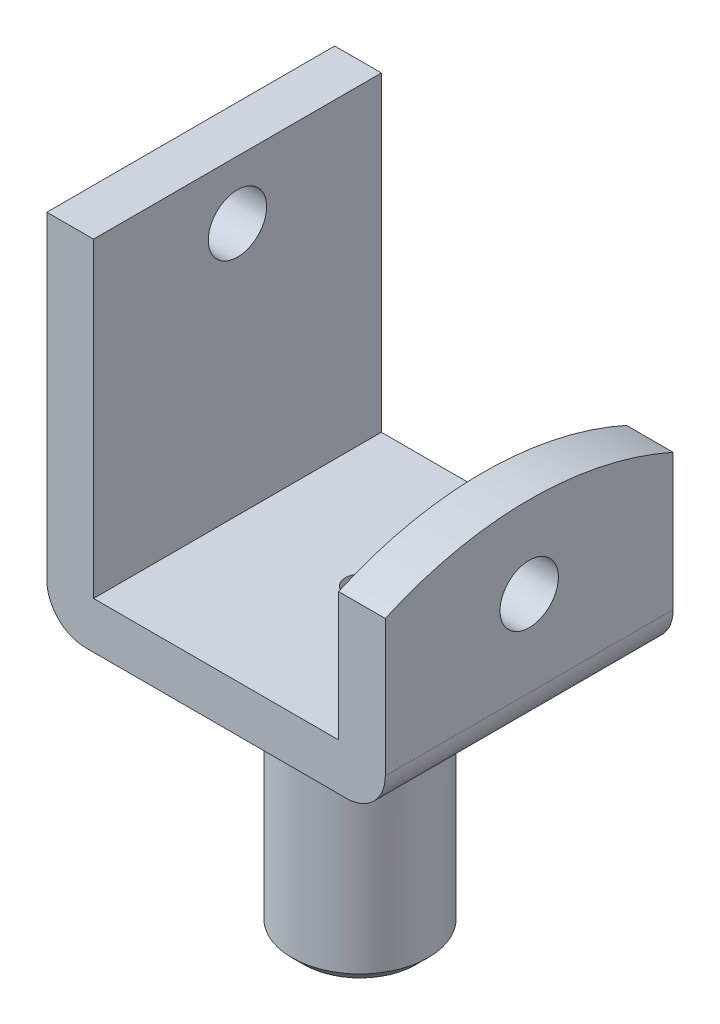
ISO-10303-21;
HEADER;
FILE_DESCRIPTION(('STEP AP214'),'2;1');
FILE_NAME('part.step','',(''),(''),'','','');
FILE_SCHEMA(('AUTOMOTIVE_DESIGN { 1 0 10303 214 1 1 1 1 }'));
ENDSEC;
DATA;
#1=APPLICATION_CONTEXT('core data for automotive mechanical design processes');
#2=APPLICATION_PROTOCOL_DEFINITION('international standard','automotive_design',2000,#1);
#3=PRODUCT_CONTEXT('',#1,'mechanical');
#4=PRODUCT('Part','Part','',(#3));
#5=PRODUCT_RELATED_PRODUCT_CATEGORY('part','',(#4));
#6=PRODUCT_DEFINITION_FORMATION('','',#4);
#7=PRODUCT_DEFINITION_CONTEXT('part definition',#1,'design');
#8=PRODUCT_DEFINITION('design','',#6,#7);
#9=PRODUCT_DEFINITION_SHAPE('','',#8);
#10=(LENGTH_UNIT() NAMED_UNIT(*) SI_UNIT(.MILLI.,.METRE.));
#11=(NAMED_UNIT(*) PLANE_ANGLE_UNIT() SI_UNIT($,.RADIAN.));
#12=(NAMED_UNIT(*) SI_UNIT($,.STERADIAN.) SOLID_ANGLE_UNIT());
#13=UNCERTAINTY_MEASURE_WITH_UNIT(LENGTH_MEASURE(1.E-05),#10,'distance_accuracy_value','');
#14=(GEOMETRIC_REPRESENTATION_CONTEXT(3) GLOBAL_UNCERTAINTY_ASSIGNED_CONTEXT((#13)) GLOBAL_UNIT_ASSIGNED_CONTEXT((#10,
#11,#12)) REPRESENTATION_CONTEXT('',''));
#15=CARTESIAN_POINT('',(0.,0.,0.));
#16=DIRECTION('',(0.,0.,1.));
#17=DIRECTION('',(1.,0.,0.));
#18=AXIS2_PLACEMENT_3D('',#15,#16,#17);
#19=CARTESIAN_POINT('',(43500.,6000.,37000.));
#20=DIRECTION('',(-1.,0.,0.));
#21=DIRECTION('',(0.,-1.,0.));
#22=AXIS2_PLACEMENT_3D('',#19,#20,#21);
#23=PLANE('',#22);
#24=CARTESIAN_POINT('',(43500.,26000.,-2.57175827820944E-12));
#25=DIRECTION('',(1.,0.,0.));
#26=DIRECTION('',(0.,1.,0.));
#27=AXIS2_PLACEMENT_3D('',#24,#25,#26);
#28=CIRCLE('',#27,7500.);
#29=CARTESIAN_POINT('',(43500.,33500.,-2.57175827820944E-12));
#30=VERTEX_POINT('',#29);
#31=EDGE_CURVE('E264',#30,#30,#28,.T.);
#32=ORIENTED_EDGE('',*,*,#31,.F.);
#33=EDGE_LOOP('',(#32));
#34=FACE_BOUND('',#33,.T.);
#35=CARTESIAN_POINT('',(43500.,-43000.,-1.10218211923262E-11));
#36=DIRECTION('',(1.,0.,0.));
#37=DIRECTION('',(0.,1.,0.));
#38=AXIS2_PLACEMENT_3D('',#35,#36,#37);
#39=CIRCLE('',#38,90000.);
#40=CARTESIAN_POINT('',(43500.,39042.6718238747,-37000.));
#41=VERTEX_POINT('',#40);
#42=CARTESIAN_POINT('',(43500.,39042.6718238747,37000.));
#43=VERTEX_POINT('',#42);
#44=EDGE_CURVE('E61',#41,#43,#39,.T.);
#45=ORIENTED_EDGE('',*,*,#44,.T.);
#46=DIRECTION('',(0.,1.,0.));
#47=VECTOR('',#46,1.);
#48=CARTESIAN_POINT('',(43500.,6000.,37000.));
#49=LINE('',#48,#47);
#50=CARTESIAN_POINT('',(43500.,4000.,37000.));
#51=VERTEX_POINT('',#50);
#52=EDGE_CURVE('E142',#51,#43,#49,.T.);
#53=ORIENTED_EDGE('',*,*,#52,.F.);
#54=DIRECTION('',(0.,0.,-1.));
#55=VECTOR('',#54,1.);
#56=CARTESIAN_POINT('',(43500.,4000.,37000.));
#57=LINE('',#56,#55);
#58=CARTESIAN_POINT('',(43500.,4000.,-37000.));
#59=VERTEX_POINT('',#58);
#60=EDGE_CURVE('E187',#51,#59,#57,.T.);
#61=ORIENTED_EDGE('',*,*,#60,.T.);
#62=DIRECTION('',(0.,1.,0.));
#63=VECTOR('',#62,1.);
#64=CARTESIAN_POINT('',(43500.,6000.,-37000.));
#65=LINE('',#64,#63);
#66=EDGE_CURVE('E162',#59,#41,#65,.T.);
#67=ORIENTED_EDGE('',*,*,#66,.T.);
#68=EDGE_LOOP('',(#45,#53,#61,#67));
#69=FACE_BOUND('',#68,.T.);
#70=ADVANCED_FACE('F48',(#34,#69),#23,.F.);
#71=CARTESIAN_POINT('',(31500.,6000.,37000.));
#72=DIRECTION('',(1.,0.,0.));
#73=DIRECTION('',(0.,0.,-1.));
#74=AXIS2_PLACEMENT_3D('',#71,#72,#73);
#75=PLANE('',#74);
#76=CARTESIAN_POINT('',(31500.,26000.,-2.57175827820944E-12));
#77=DIRECTION('',(1.,0.,0.));
#78=DIRECTION('',(0.,1.,0.));
#79=AXIS2_PLACEMENT_3D('',#76,#77,#78);
#80=CIRCLE('',#79,7500.);
#81=CARTESIAN_POINT('',(31500.,33500.,-2.57175827820944E-12));
#82=VERTEX_POINT('',#81);
#83=EDGE_CURVE('E263',#82,#82,#80,.T.);
#84=ORIENTED_EDGE('',*,*,#83,.T.);
#85=EDGE_LOOP('',(#84));
#86=FACE_BOUND('',#85,.T.);
#87=CARTESIAN_POINT('',(31500.,-43000.,-1.10218211923262E-11));
#88=DIRECTION('',(1.,0.,0.));
#89=DIRECTION('',(0.,1.,0.));
#90=AXIS2_PLACEMENT_3D('',#87,#88,#89);
#91=CIRCLE('',#90,90000.);
#92=CARTESIAN_POINT('',(31500.,39042.6718238747,-37000.));
#93=VERTEX_POINT('',#92);
#94=CARTESIAN_POINT('',(31500.,39042.6718238747,37000.));
#95=VERTEX_POINT('',#94);
#96=EDGE_CURVE('E127',#93,#95,#91,.T.);
#97=ORIENTED_EDGE('',*,*,#96,.F.);
#98=DIRECTION('',(0.,-1.,0.));
#99=VECTOR('',#98,1.);
#100=CARTESIAN_POINT('',(31500.,6000.,-37000.));
#101=LINE('',#100,#99);
#102=CARTESIAN_POINT('',(31500.,6000.,-37000.));
#103=VERTEX_POINT('',#102);
#104=EDGE_CURVE('E164',#93,#103,#101,.T.);
#105=ORIENTED_EDGE('',*,*,#104,.T.);
#106=DIRECTION('',(0.,0.,-1.));
#107=VECTOR('',#106,1.);
#108=CARTESIAN_POINT('',(31500.,6000.,37000.));
#109=LINE('',#108,#107);
#110=CARTESIAN_POINT('',(31500.,6000.,37000.));
#111=VERTEX_POINT('',#110);
#112=EDGE_CURVE('E143',#111,#103,#109,.T.);
#113=ORIENTED_EDGE('',*,*,#112,.F.);
#114=DIRECTION('',(0.,-1.,0.));
#115=VECTOR('',#114,1.);
#116=CARTESIAN_POINT('',(31500.,6000.,37000.));
#117=LINE('',#116,#115);
#118=EDGE_CURVE('E140',#95,#111,#117,.T.);
#119=ORIENTED_EDGE('',*,*,#118,.F.);
#120=EDGE_LOOP('',(#97,#105,#113,#119));
#121=FACE_BOUND('',#120,.T.);
#122=ADVANCED_FACE('F141',(#86,#121),#75,.F.);
#123=CARTESIAN_POINT('',(0.,0.,37000.));
#124=DIRECTION('',(0.,0.,1.));
#125=DIRECTION('',(1.,0.,0.));
#126=AXIS2_PLACEMENT_3D('',#123,#124,#125);
#127=PLANE('',#126);
#128=ORIENTED_EDGE('',*,*,#118,.T.);
#129=DIRECTION('',(-1.,0.,0.));
#130=VECTOR('',#129,1.);
#131=CARTESIAN_POINT('',(-31500.,5999.99999999999,37000.));
#132=LINE('',#131,#130);
#133=CARTESIAN_POINT('',(-31500.,5999.99999999999,37000.));
#134=VERTEX_POINT('',#133);
#135=EDGE_CURVE('E150',#111,#134,#132,.T.);
#136=ORIENTED_EDGE('',*,*,#135,.T.);
#137=DIRECTION('',(0.,1.,0.));
#138=VECTOR('',#137,1.);
#139=CARTESIAN_POINT('',(-31500.,5999.99999999999,37000.));
#140=LINE('',#139,#138);
#141=CARTESIAN_POINT('',(-31500.,86000.,37000.));
#142=VERTEX_POINT('',#141);
#143=EDGE_CURVE('E146',#134,#142,#140,.T.);
#144=ORIENTED_EDGE('',*,*,#143,.T.);
#145=DIRECTION('',(-1.,0.,0.));
#146=VECTOR('',#145,1.);
#147=CARTESIAN_POINT('',(-43500.,86000.,37000.));
#148=LINE('',#147,#146);
#149=CARTESIAN_POINT('',(-43500.,86000.,37000.));
#150=VERTEX_POINT('',#149);
#151=EDGE_CURVE('E152',#142,#150,#148,.T.);
#152=ORIENTED_EDGE('',*,*,#151,.T.);
#153=DIRECTION('',(0.,-1.,0.));
#154=VECTOR('',#153,1.);
#155=CARTESIAN_POINT('',(-43500.,6000.,37000.));
#156=LINE('',#155,#154);
#157=CARTESIAN_POINT('',(-43500.,4000.,37000.));
#158=VERTEX_POINT('',#157);
#159=EDGE_CURVE('E159',#150,#158,#156,.T.);
#160=ORIENTED_EDGE('',*,*,#159,.T.);
#161=CARTESIAN_POINT('',(-33500.,4000.,37000.));
#162=DIRECTION('',(0.,0.,1.));
#163=DIRECTION('',(1.,0.,0.));
#164=AXIS2_PLACEMENT_3D('',#161,#162,#163);
#165=CIRCLE('',#164,10000.);
#166=CARTESIAN_POINT('',(-33500.,-6000.,37000.));
#167=VERTEX_POINT('',#166);
#168=EDGE_CURVE('E205',#158,#167,#165,.T.);
#169=ORIENTED_EDGE('',*,*,#168,.T.);
#170=DIRECTION('',(1.,0.,0.));
#171=VECTOR('',#170,1.);
#172=CARTESIAN_POINT('',(-43500.,-6000.,37000.));
#173=LINE('',#172,#171);
#174=CARTESIAN_POINT('',(33500.,-6000.,37000.));
#175=VERTEX_POINT('',#174);
#176=EDGE_CURVE('E156',#167,#175,#173,.T.);
#177=ORIENTED_EDGE('',*,*,#176,.T.);
#178=CARTESIAN_POINT('',(33500.,4000.,37000.));
#179=DIRECTION('',(0.,0.,1.));
#180=DIRECTION('',(1.,0.,0.));
#181=AXIS2_PLACEMENT_3D('',#178,#179,#180);
#182=CIRCLE('',#181,10000.);
#183=EDGE_CURVE('E193',#175,#51,#182,.T.);
#184=ORIENTED_EDGE('',*,*,#183,.T.);
#185=ORIENTED_EDGE('',*,*,#52,.T.);
#186=DIRECTION('',(1.,0.,0.));
#187=VECTOR('',#186,1.);
#188=CARTESIAN_POINT('',(31500.,39042.6718238747,37000.));
#189=LINE('',#188,#187);
#190=EDGE_CURVE('E126',#95,#43,#189,.T.);
#191=ORIENTED_EDGE('',*,*,#190,.F.);
#192=EDGE_LOOP('',(#128,#136,#144,#152,#160,#169,#177,#184,#185,#191));
#193=FACE_BOUND('',#192,.T.);
#194=ADVANCED_FACE('F139',(#193),#127,.T.);
#195=CARTESIAN_POINT('',(0.,0.,-37000.));
#196=DIRECTION('',(0.,0.,1.));
#197=DIRECTION('',(1.,0.,0.));
#198=AXIS2_PLACEMENT_3D('',#195,#196,#197);
#199=PLANE('',#198);
#200=CARTESIAN_POINT('',(33500.,4000.,-37000.));
#201=DIRECTION('',(0.,0.,1.));
#202=DIRECTION('',(1.,0.,0.));
#203=AXIS2_PLACEMENT_3D('',#200,#201,#202);
#204=CIRCLE('',#203,10000.);
#205=CARTESIAN_POINT('',(33500.,-6000.,-37000.));
#206=VERTEX_POINT('',#205);
#207=EDGE_CURVE('E186',#59,#206,#204,.F.);
#208=ORIENTED_EDGE('',*,*,#207,.T.);
#209=DIRECTION('',(1.,0.,0.));
#210=VECTOR('',#209,1.);
#211=CARTESIAN_POINT('',(-43500.,-6000.,-37000.));
#212=LINE('',#211,#210);
#213=CARTESIAN_POINT('',(-33500.,-6000.,-37000.));
#214=VERTEX_POINT('',#213);
#215=EDGE_CURVE('E153',#214,#206,#212,.T.);
#216=ORIENTED_EDGE('',*,*,#215,.F.);
#217=CARTESIAN_POINT('',(-33500.,4000.,-37000.));
#218=DIRECTION('',(0.,0.,1.));
#219=DIRECTION('',(1.,0.,0.));
#220=AXIS2_PLACEMENT_3D('',#217,#218,#219);
#221=CIRCLE('',#220,10000.);
#222=CARTESIAN_POINT('',(-43500.,4000.,-37000.));
#223=VERTEX_POINT('',#222);
#224=EDGE_CURVE('E197',#214,#223,#221,.F.);
#225=ORIENTED_EDGE('',*,*,#224,.T.);
#226=DIRECTION('',(0.,-1.,0.));
#227=VECTOR('',#226,1.);
#228=CARTESIAN_POINT('',(-43500.,6000.,-37000.));
#229=LINE('',#228,#227);
#230=CARTESIAN_POINT('',(-43500.,86000.,-37000.));
#231=VERTEX_POINT('',#230);
#232=EDGE_CURVE('E172',#231,#223,#229,.T.);
#233=ORIENTED_EDGE('',*,*,#232,.F.);
#234=DIRECTION('',(-1.,0.,0.));
#235=VECTOR('',#234,1.);
#236=CARTESIAN_POINT('',(-43500.,86000.,-37000.));
#237=LINE('',#236,#235);
#238=CARTESIAN_POINT('',(-31500.,86000.,-37000.));
#239=VERTEX_POINT('',#238);
#240=EDGE_CURVE('E171',#239,#231,#237,.T.);
#241=ORIENTED_EDGE('',*,*,#240,.F.);
#242=DIRECTION('',(0.,1.,0.));
#243=VECTOR('',#242,1.);
#244=CARTESIAN_POINT('',(-31500.,5999.99999999999,-37000.));
#245=LINE('',#244,#243);
#246=CARTESIAN_POINT('',(-31500.,5999.99999999999,-37000.));
#247=VERTEX_POINT('',#246);
#248=EDGE_CURVE('E169',#247,#239,#245,.T.);
#249=ORIENTED_EDGE('',*,*,#248,.F.);
#250=DIRECTION('',(-1.,0.,0.));
#251=VECTOR('',#250,1.);
#252=CARTESIAN_POINT('',(-31500.,5999.99999999999,-37000.));
#253=LINE('',#252,#251);
#254=EDGE_CURVE('E170',#103,#247,#253,.T.);
#255=ORIENTED_EDGE('',*,*,#254,.F.);
#256=ORIENTED_EDGE('',*,*,#104,.F.);
#257=DIRECTION('',(1.,0.,0.));
#258=VECTOR('',#257,1.);
#259=CARTESIAN_POINT('',(31500.,39042.6718238747,-37000.));
#260=LINE('',#259,#258);
#261=EDGE_CURVE('E133',#93,#41,#260,.T.);
#262=ORIENTED_EDGE('',*,*,#261,.T.);
#263=ORIENTED_EDGE('',*,*,#66,.F.);
#264=EDGE_LOOP('',(#208,#216,#225,#233,#241,#249,#255,#256,#262,#263));
#265=FACE_BOUND('',#264,.T.);
#266=ADVANCED_FACE('F266',(#265),#199,.F.);
#267=CARTESIAN_POINT('',(-31500.,5999.99999999999,37000.));
#268=DIRECTION('',(0.,-1.,0.));
#269=DIRECTION('',(1.,0.,0.));
#270=AXIS2_PLACEMENT_3D('',#267,#268,#269);
#271=PLANE('',#270);
#272=CARTESIAN_POINT('',(0.,5999.99999999999,0.));
#273=DIRECTION('',(0.,-1.,0.));
#274=DIRECTION('',(1.,0.,0.));
#275=AXIS2_PLACEMENT_3D('',#272,#273,#274);
#276=CIRCLE('',#275,3750.);
#277=CARTESIAN_POINT('',(3750.,5999.99999999999,0.));
#278=VERTEX_POINT('',#277);
#279=EDGE_CURVE('E310',#278,#278,#276,.T.);
#280=ORIENTED_EDGE('',*,*,#279,.T.);
#281=EDGE_LOOP('',(#280));
#282=FACE_BOUND('',#281,.T.);
#283=ORIENTED_EDGE('',*,*,#254,.T.);
#284=DIRECTION('',(0.,0.,-1.));
#285=VECTOR('',#284,1.);
#286=CARTESIAN_POINT('',(-31500.,5999.99999999999,37000.));
#287=LINE('',#286,#285);
#288=EDGE_CURVE('E185',#134,#247,#287,.T.);
#289=ORIENTED_EDGE('',*,*,#288,.F.);
#290=ORIENTED_EDGE('',*,*,#135,.F.);
#291=ORIENTED_EDGE('',*,*,#112,.T.);
#292=EDGE_LOOP('',(#283,#289,#290,#291));
#293=FACE_BOUND('',#292,.T.);
#294=ADVANCED_FACE('F271',(#282,#293),#271,.F.);
#295=CARTESIAN_POINT('',(-31500.,5999.99999999999,37000.));
#296=DIRECTION('',(-1.,0.,0.));
#297=DIRECTION('',(0.,0.,1.));
#298=AXIS2_PLACEMENT_3D('',#295,#296,#297);
#299=PLANE('',#298);
#300=CARTESIAN_POINT('',(-31500.,71000.,1.83697019872103E-12));
#301=DIRECTION('',(-1.,0.,0.));
#302=DIRECTION('',(0.,0.,1.));
#303=AXIS2_PLACEMENT_3D('',#300,#301,#302);
#304=CIRCLE('',#303,7500.);
#305=CARTESIAN_POINT('',(-31500.,71000.,7500.));
#306=VERTEX_POINT('',#305);
#307=EDGE_CURVE('E312',#306,#306,#304,.T.);
#308=ORIENTED_EDGE('',*,*,#307,.T.);
#309=EDGE_LOOP('',(#308));
#310=FACE_BOUND('',#309,.T.);
#311=ORIENTED_EDGE('',*,*,#248,.T.);
#312=DIRECTION('',(0.,0.,-1.));
#313=VECTOR('',#312,1.);
#314=CARTESIAN_POINT('',(-31500.,86000.,37000.));
#315=LINE('',#314,#313);
#316=EDGE_CURVE('E177',#142,#239,#315,.T.);
#317=ORIENTED_EDGE('',*,*,#316,.F.);
#318=ORIENTED_EDGE('',*,*,#143,.F.);
#319=ORIENTED_EDGE('',*,*,#288,.T.);
#320=EDGE_LOOP('',(#311,#317,#318,#319));
#321=FACE_BOUND('',#320,.T.);
#322=ADVANCED_FACE('F278',(#310,#321),#299,.F.);
#323=CARTESIAN_POINT('',(-43500.,86000.,37000.));
#324=DIRECTION('',(0.,-1.,0.));
#325=DIRECTION('',(0.,0.,-1.));
#326=AXIS2_PLACEMENT_3D('',#323,#324,#325);
#327=PLANE('',#326);
#328=ORIENTED_EDGE('',*,*,#240,.T.);
#329=DIRECTION('',(0.,0.,-1.));
#330=VECTOR('',#329,1.);
#331=CARTESIAN_POINT('',(-43500.,86000.,37000.));
#332=LINE('',#331,#330);
#333=EDGE_CURVE('E163',#150,#231,#332,.T.);
#334=ORIENTED_EDGE('',*,*,#333,.F.);
#335=ORIENTED_EDGE('',*,*,#151,.F.);
#336=ORIENTED_EDGE('',*,*,#316,.T.);
#337=EDGE_LOOP('',(#328,#334,#335,#336));
#338=FACE_BOUND('',#337,.T.);
#339=ADVANCED_FACE('F281',(#338),#327,.F.);
#340=CARTESIAN_POINT('',(-43500.,6000.,37000.));
#341=DIRECTION('',(1.,0.,0.));
#342=DIRECTION('',(0.,0.,-1.));
#343=AXIS2_PLACEMENT_3D('',#340,#341,#342);
#344=PLANE('',#343);
#345=CARTESIAN_POINT('',(-43500.,71000.,1.83697019872103E-12));
#346=DIRECTION('',(-1.,0.,0.));
#347=DIRECTION('',(0.,0.,1.));
#348=AXIS2_PLACEMENT_3D('',#345,#346,#347);
#349=CIRCLE('',#348,7500.);
#350=CARTESIAN_POINT('',(-43500.,71000.,7500.));
#351=VERTEX_POINT('',#350);
#352=EDGE_CURVE('E307',#351,#351,#349,.T.);
#353=ORIENTED_EDGE('',*,*,#352,.F.);
#354=EDGE_LOOP('',(#353));
#355=FACE_BOUND('',#354,.T.);
#356=ORIENTED_EDGE('',*,*,#232,.T.);
#357=DIRECTION('',(0.,0.,-1.));
#358=VECTOR('',#357,1.);
#359=CARTESIAN_POINT('',(-43500.,4000.,37000.));
#360=LINE('',#359,#358);
#361=EDGE_CURVE('E74',#223,#158,#360,.F.);
#362=ORIENTED_EDGE('',*,*,#361,.T.);
#363=ORIENTED_EDGE('',*,*,#159,.F.);
#364=ORIENTED_EDGE('',*,*,#333,.T.);
#365=EDGE_LOOP('',(#356,#362,#363,#364));
#366=FACE_BOUND('',#365,.T.);
#367=ADVANCED_FACE('F284',(#355,#366),#344,.F.);
#368=CARTESIAN_POINT('',(-43500.,-6000.,37000.));
#369=DIRECTION('',(0.,1.,0.));
#370=DIRECTION('',(0.,0.,1.));
#371=AXIS2_PLACEMENT_3D('',#368,#369,#370);
#372=PLANE('',#371);
#373=CARTESIAN_POINT('',(0.,-6000.,0.));
#374=DIRECTION('',(0.,1.,0.));
#375=DIRECTION('',(0.,0.,1.));
#376=AXIS2_PLACEMENT_3D('',#373,#374,#375);
#377=CIRCLE('',#376,22500.);
#378=CARTESIAN_POINT('',(0.,-6000.,22500.));
#379=VERTEX_POINT('',#378);
#380=EDGE_CURVE('E206',#379,#379,#377,.T.);
#381=ORIENTED_EDGE('',*,*,#380,.T.);
#382=EDGE_LOOP('',(#381));
#383=FACE_BOUND('',#382,.T.);
#384=DIRECTION('',(0.,0.,-1.));
#385=VECTOR('',#384,1.);
#386=CARTESIAN_POINT('',(33500.,-6000.,37000.));
#387=LINE('',#386,#385);
#388=EDGE_CURVE('E195',#206,#175,#387,.F.);
#389=ORIENTED_EDGE('',*,*,#388,.T.);
#390=ORIENTED_EDGE('',*,*,#176,.F.);
#391=DIRECTION('',(0.,0.,-1.));
#392=VECTOR('',#391,1.);
#393=CARTESIAN_POINT('',(-33500.,-6000.,37000.));
#394=LINE('',#393,#392);
#395=EDGE_CURVE('E200',#167,#214,#394,.T.);
#396=ORIENTED_EDGE('',*,*,#395,.T.);
#397=ORIENTED_EDGE('',*,*,#215,.T.);
#398=EDGE_LOOP('',(#389,#390,#396,#397));
#399=FACE_BOUND('',#398,.T.);
#400=ADVANCED_FACE('F243',(#383,#399),#372,.F.);
#401=CARTESIAN_POINT('',(33500.,4000.,37000.));
#402=DIRECTION('',(0.,0.,-1.));
#403=DIRECTION('',(-1.,0.,0.));
#404=AXIS2_PLACEMENT_3D('',#401,#402,#403);
#405=CYLINDRICAL_SURFACE('',#404,10000.);
#406=ORIENTED_EDGE('',*,*,#183,.F.);
#407=ORIENTED_EDGE('',*,*,#388,.F.);
#408=ORIENTED_EDGE('',*,*,#207,.F.);
#409=ORIENTED_EDGE('',*,*,#60,.F.);
#410=EDGE_LOOP('',(#406,#407,#408,#409));
#411=FACE_BOUND('',#410,.T.);
#412=ADVANCED_FACE('F237',(#411),#405,.T.);
#413=CARTESIAN_POINT('',(-33500.,4000.,37000.));
#414=DIRECTION('',(0.,0.,-1.));
#415=DIRECTION('',(-1.,0.,0.));
#416=AXIS2_PLACEMENT_3D('',#413,#414,#415);
#417=CYLINDRICAL_SURFACE('',#416,10000.);
#418=ORIENTED_EDGE('',*,*,#168,.F.);
#419=ORIENTED_EDGE('',*,*,#361,.F.);
#420=ORIENTED_EDGE('',*,*,#224,.F.);
#421=ORIENTED_EDGE('',*,*,#395,.F.);
#422=EDGE_LOOP('',(#418,#419,#420,#421));
#423=FACE_BOUND('',#422,.T.);
#424=ADVANCED_FACE('F245',(#423),#417,.T.);
#425=CARTESIAN_POINT('',(31500.,-43000.,-1.10218211923262E-11));
#426=DIRECTION('',(1.,0.,0.));
#427=DIRECTION('',(0.,1.,0.));
#428=AXIS2_PLACEMENT_3D('',#425,#426,#427);
#429=CYLINDRICAL_SURFACE('',#428,90000.);
#430=ORIENTED_EDGE('',*,*,#96,.T.);
#431=ORIENTED_EDGE('',*,*,#190,.T.);
#432=ORIENTED_EDGE('',*,*,#44,.F.);
#433=ORIENTED_EDGE('',*,*,#261,.F.);
#434=EDGE_LOOP('',(#430,#431,#432,#433));
#435=FACE_BOUND('',#434,.T.);
#436=ADVANCED_FACE('F129',(#435),#429,.T.);
#437=CARTESIAN_POINT('',(31500.,26000.,-2.57175827820944E-12));
#438=DIRECTION('',(1.,0.,0.));
#439=DIRECTION('',(0.,1.,0.));
#440=AXIS2_PLACEMENT_3D('',#437,#438,#439);
#441=CYLINDRICAL_SURFACE('',#440,7500.);
#442=ORIENTED_EDGE('',*,*,#83,.F.);
#443=EDGE_LOOP('',(#442));
#444=FACE_BOUND('',#443,.T.);
#445=ORIENTED_EDGE('',*,*,#31,.T.);
#446=EDGE_LOOP('',(#445));
#447=FACE_BOUND('',#446,.T.);
#448=ADVANCED_FACE('F249',(#444,#447),#441,.F.);
#449=CARTESIAN_POINT('',(-31500.,71000.,1.83697019872103E-12));
#450=DIRECTION('',(-1.,0.,0.));
#451=DIRECTION('',(0.,0.,1.));
#452=AXIS2_PLACEMENT_3D('',#449,#450,#451);
#453=CYLINDRICAL_SURFACE('',#452,7500.);
#454=ORIENTED_EDGE('',*,*,#307,.F.);
#455=EDGE_LOOP('',(#454));
#456=FACE_BOUND('',#455,.T.);
#457=ORIENTED_EDGE('',*,*,#352,.T.);
#458=EDGE_LOOP('',(#457));
#459=FACE_BOUND('',#458,.T.);
#460=ADVANCED_FACE('F325',(#456,#459),#453,.F.);
#461=CARTESIAN_POINT('',(0.,-71000.,0.));
#462=DIRECTION('',(0.,1.,0.));
#463=DIRECTION('',(0.,0.,1.));
#464=AXIS2_PLACEMENT_3D('',#461,#462,#463);
#465=CYLINDRICAL_SURFACE('',#464,17500.);
#466=CARTESIAN_POINT('',(0.,-68000.,0.));
#467=DIRECTION('',(0.,-1.,0.));
#468=DIRECTION('',(0.,0.,-1.));
#469=AXIS2_PLACEMENT_3D('',#466,#467,#468);
#470=CIRCLE('',#469,17500.);
#471=CARTESIAN_POINT('',(0.,-68000.,-17500.));
#472=VERTEX_POINT('',#471);
#473=EDGE_CURVE('E12',#472,#472,#470,.F.);
#474=ORIENTED_EDGE('',*,*,#473,.T.);
#475=EDGE_LOOP('',(#474));
#476=FACE_BOUND('',#475,.T.);
#477=CARTESIAN_POINT('',(0.,-11000.,0.));
#478=DIRECTION('',(0.,1.,0.));
#479=DIRECTION('',(0.,0.,1.));
#480=AXIS2_PLACEMENT_3D('',#477,#478,#479);
#481=CIRCLE('',#480,17500.);
#482=CARTESIAN_POINT('',(0.,-11000.,17500.));
#483=VERTEX_POINT('',#482);
#484=EDGE_CURVE('E203',#483,#483,#481,.F.);
#485=ORIENTED_EDGE('',*,*,#484,.T.);
#486=EDGE_LOOP('',(#485));
#487=FACE_BOUND('',#486,.T.);
#488=ADVANCED_FACE('F326',(#476,#487),#465,.T.);
#489=CARTESIAN_POINT('',(0.,-71000.,0.));
#490=DIRECTION('',(0.,-1.,0.));
#491=DIRECTION('',(0.,0.,-1.));
#492=AXIS2_PLACEMENT_3D('',#489,#490,#491);
#493=PLANE('',#492);
#494=CARTESIAN_POINT('',(0.,-71000.,0.));
#495=DIRECTION('',(0.,-1.,0.));
#496=DIRECTION('',(0.,0.,-1.));
#497=AXIS2_PLACEMENT_3D('',#494,#495,#496);
#498=CIRCLE('',#497,3750.);
#499=CARTESIAN_POINT('',(0.,-71000.,-3750.));
#500=VERTEX_POINT('',#499);
#501=EDGE_CURVE('E309',#500,#500,#498,.T.);
#502=ORIENTED_EDGE('',*,*,#501,.F.);
#503=EDGE_LOOP('',(#502));
#504=FACE_BOUND('',#503,.T.);
#505=CARTESIAN_POINT('',(0.,-71000.,0.));
#506=DIRECTION('',(0.,-1.,0.));
#507=DIRECTION('',(0.,0.,-1.));
#508=AXIS2_PLACEMENT_3D('',#505,#506,#507);
#509=CIRCLE('',#508,14500.);
#510=CARTESIAN_POINT('',(0.,-71000.,-14500.));
#511=VERTEX_POINT('',#510);
#512=EDGE_CURVE('E60',#511,#511,#509,.T.);
#513=ORIENTED_EDGE('',*,*,#512,.T.);
#514=EDGE_LOOP('',(#513));
#515=FACE_BOUND('',#514,.T.);
#516=ADVANCED_FACE('F214',(#504,#515),#493,.T.);
#517=CARTESIAN_POINT('',(0.,-11000.,0.));
#518=DIRECTION('',(0.,1.,0.));
#519=DIRECTION('',(0.,0.,1.));
#520=AXIS2_PLACEMENT_3D('',#517,#518,#519);
#521=TOROIDAL_SURFACE('',#520,22500.,5000.);
#522=ORIENTED_EDGE('',*,*,#380,.F.);
#523=EDGE_LOOP('',(#522));
#524=FACE_BOUND('',#523,.T.);
#525=ORIENTED_EDGE('',*,*,#484,.F.);
#526=EDGE_LOOP('',(#525));
#527=FACE_BOUND('',#526,.T.);
#528=ADVANCED_FACE('F220',(#524,#527),#521,.F.);
#529=CARTESIAN_POINT('',(0.,-71000.,0.));
#530=DIRECTION('',(0.,1.,0.));
#531=DIRECTION('',(0.,0.,1.));
#532=AXIS2_PLACEMENT_3D('',#529,#530,#531);
#533=CONICAL_SURFACE('',#532,14500.,0.785398163397453);
#534=ORIENTED_EDGE('',*,*,#473,.F.);
#535=EDGE_LOOP('',(#534));
#536=FACE_BOUND('',#535,.T.);
#537=ORIENTED_EDGE('',*,*,#512,.F.);
#538=EDGE_LOOP('',(#537));
#539=FACE_BOUND('',#538,.T.);
#540=ADVANCED_FACE('F51',(#536,#539),#533,.T.);
#541=CARTESIAN_POINT('',(0.,86000.,0.));
#542=DIRECTION('',(0.,-1.,0.));
#543=DIRECTION('',(0.,0.,-1.));
#544=AXIS2_PLACEMENT_3D('',#541,#542,#543);
#545=CYLINDRICAL_SURFACE('',#544,3750.);
#546=ORIENTED_EDGE('',*,*,#501,.T.);
#547=EDGE_LOOP('',(#546));
#548=FACE_BOUND('',#547,.T.);
#549=ORIENTED_EDGE('',*,*,#279,.F.);
#550=EDGE_LOOP('',(#549));
#551=FACE_BOUND('',#550,.T.);
#552=ADVANCED_FACE('F218',(#548,#551),#545,.F.);
#553=CLOSED_SHELL('',(#70,#122,#194,#266,#294,#322,#339,#367,#400,#412,#424,#436,#448,#460,#488,
#516,#528,#540,#552));
#554=MANIFOLD_SOLID_BREP('B2',#553);
#555=ADVANCED_BREP_SHAPE_REPRESENTATION('',(#18,#554),#14);
#556=SHAPE_DEFINITION_REPRESENTATION(#9,#555);
ENDSEC;
END-ISO-10303-21;
